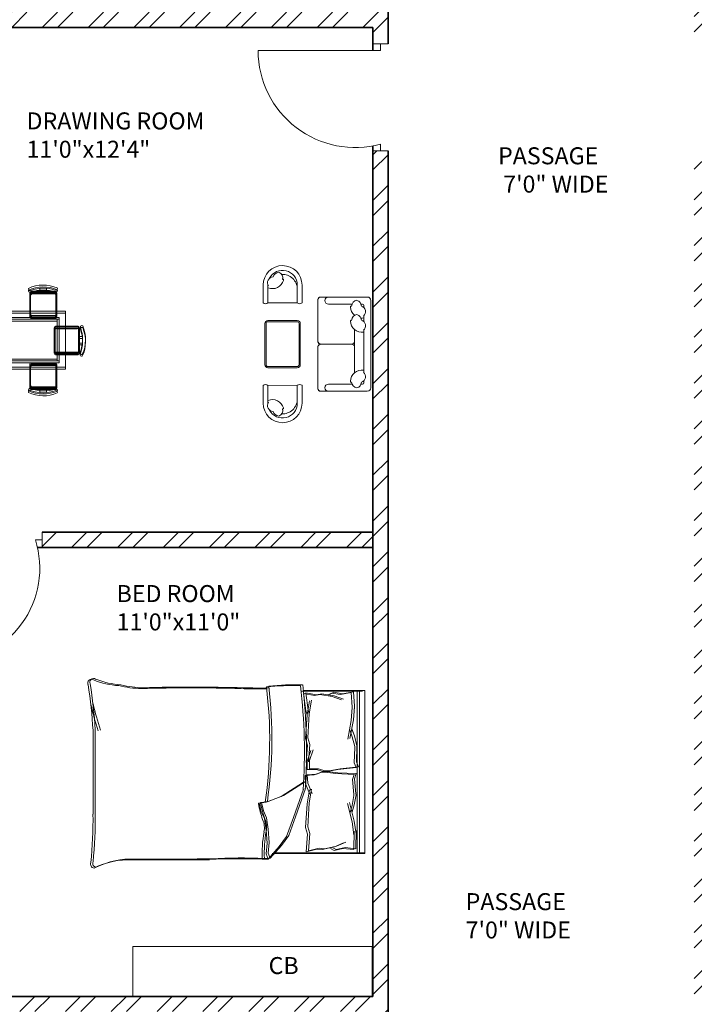
# Model space of a CAD drawing. Units: inches. Extents: x 2168 to 3056, y 1130 to 2629.
# Tile 5 of 42: x 2447 to 2645, y 1789 to 2079. Entities that reach past the tile are written whole.
import ezdxf

# ---------------------------------------------------------------- set-up
doc = ezdxf.new("R2010")
doc.units = ezdxf.units.IN
for name, color, linetype, lineweight in [('A-ANNO-TEXT', 7, 'Continuous', 18), ('A-AREA-IDEN', 7, 'Continuous', 18), ('A-DOOR', 21, 'Continuous', 18), ('A-FLOR-CASE', 71, 'Continuous', 18), ('A-FURN', 8, 'Continuous', 13), ('A-WALL', 7, 'Continuous', 35)]:
    doc.layers.add(name, color=color, linetype=linetype, lineweight=lineweight)
doc.layers.add('A-WALL-PATT', color=143, linetype='Continuous', lineweight=13, true_color=0x7aafdf)
doc.styles.get("Standard").update_dxf_attribs({"font": 'arial.ttf'})

# ---------------------------------------------------------------- blocks, each defined once
blk = doc.blocks.new('A$C1352')
at = {"color": 0}
for points in [[(0.003, 0.053), (0.003, 0.553, -0.414214), (0.053, 0.603), (0.753, 0.603, -0.414214), (0.803, 0.553), (0.803, 0.053, -0.414214), (0.753, 0.003), (0.053, 0.003, -0.414214)], [(0.023, 0.053), (0.023, 0.553, -0.414214), (0.053, 0.583), (0.753, 0.583, -0.414214), (0.783, 0.553), (0.783, 0.053, -0.414214), (0.753, 0.023), (0.053, 0.023, -0.414214)]]:
    blk.add_lwpolyline(points, format="xyb", close=True, dxfattribs=at)
blk = doc.blocks.new('BED-DOUBLE')
for p, q in [((27.75, 52.87), (24.5, 49.16)), ((27.75, 52.87), (24.5, 49.16)), ((28.39, 53.1), (25.14, 49.39)), ((28.39, 53.1), (25.14, 49.39)), ((29.49, 52.95), (27.75, 52.87, 3.87)), ((29.49, 52.95), (27.75, 52.87, 3.87)), ((28.37, 51.33), (27.75, 52.87)), ((28.37, 51.33), (27.75, 52.87)), ((30.13, 53.18), (28.39, 53.1, 3.87)), ((30.13, 53.18), (28.39, 53.1, 3.87)), ((29, 51.56), (28.39, 53.1)), ((29, 51.56), (28.39, 53.1)), ((0, 51.49), (0.64, 51.49)), ((0, 3.48), (0, 51.49)), ((0, 51.27), (26.61, 51.27)), ((0, 51.27), (26.61, 51.27)), ((0.64, 51.49), (27.25, 51.49)), ((0.64, 51.49), (27.25, 51.49)), ((1.53, 3.48), (1.53, 51.27)), ((1.53, 3.48), (1.53, 51.27)), ((2.17, 3.7), (2.17, 51.49)), ((2.17, 3.7), (2.17, 51.49)), ((2.56, 50.11), (2.46, 44.71)), ((2.56, 50.11), (2.46, 44.71)), ((2.56, 50.11), (5.77, 49.73)), ((2.56, 50.11), (5.77, 49.73)), ((3.2, 50.34), (3.1, 44.94)), ((3.2, 50.34), (3.1, 44.94)), ((3.2, 50.34), (6.41, 49.96)), ((3.2, 50.34), (6.41, 49.96)), ((8.26, 49.31), (5.58, 48.13)), ((8.26, 49.31), (5.58, 48.13)), ((5.77, 49.73), (8.34, 50.33)), ((5.77, 49.73), (8.34, 50.33)), ((8.9, 49.54), (6.22, 48.36)), ((8.9, 49.54), (6.22, 48.36)), ((6.41, 49.96), (8.98, 50.56)), ((6.41, 49.96), (8.98, 50.56)), ((11.83, 50.11), (8.26, 49.31)), ((11.83, 50.11), (8.26, 49.31)), ((8.34, 50.33), (9.38, 49.81)), ((8.34, 50.33), (9.38, 49.81)), ((12.47, 50.34), (8.9, 49.54)), ((12.47, 50.34), (8.9, 49.54)), ((8.98, 50.56), (10.02, 50.04)), ((8.98, 50.56), (10.02, 50.04)), ((13.43, 49.92), (11.83, 50.11)), ((13.43, 49.92), (11.83, 50.11)), ((14.07, 50.15), (12.47, 50.34)), ((14.07, 50.15), (12.47, 50.34)), ((16.57, 50.7), (13.43, 49.92)), ((16.57, 50.7), (13.43, 49.92)), ((17.21, 50.93), (14.07, 50.15)), ((17.21, 50.93), (14.07, 50.15)), ((16.17, 45.57), (16.57, 50.7)), ((16.17, 45.57), (16.57, 50.7)), ((16.81, 45.8), (17.21, 50.93)), ((16.81, 45.79), (17.21, 50.93)), ((25.14, 49.39), (22.97, 46.45)), ((25.14, 49.39), (22.97, 46.45)), ((28.06, 48.23), (28.37, 51.33)), ((28.06, 48.23), (28.37, 51.33)), ((28.7, 48.46), (29, 51.56)), ((28.7, 48.46), (29, 51.56)), ((22.97, 46.45), (20.96, 40.87)), ((22.97, 46.45), (20.96, 40.87)), ((24.5, 49.16), (22.33, 46.22)), ((24.5, 49.16), (22.33, 46.22)), ((28.37, 44.36), (28.06, 48.23)), ((28.37, 44.36), (28.06, 48.23)), ((29, 44.59), (28.7, 48.46)), ((29, 44.59), (28.7, 48.46)), ((2.46, 44.71), (2.54, 45.71)), ((2.46, 44.71), (2.54, 45.71)), ((2.54, 45.71), (3.07, 41.91)), ((2.54, 45.71), (3.07, 41.91)), ((3.1, 44.94), (3.18, 45.94)), ((3.1, 44.94), (3.18, 45.94)), ((3.18, 45.94), (3.71, 42.14)), ((3.18, 45.94), (3.71, 42.14)), ((16.73, 43.61), (16.17, 45.57)), ((16.73, 43.61), (16.17, 45.57)), ((16.3, 36.6), (16.73, 43.61)), ((16.3, 36.6), (16.73, 43.61)), ((17.37, 43.83), (16.81, 45.8)), ((17.37, 43.83), (16.81, 45.79)), ((16.93, 36.82), (17.37, 43.83)), ((16.93, 36.82), (17.37, 43.83)), ((22.33, 46.22), (20.32, 40.64)), ((22.33, 46.22), (20.32, 40.64)), ((28.83, 40.95), (28.37, 44.36)), ((28.83, 40.95), (28.37, 44.36)), ((29.47, 41.18), (29, 44.59)), ((29.47, 41.18), (29, 44.59)), ((3.07, 41.91), (4.42, 36.5)), ((3.07, 41.91), (4.42, 36.49)), ((3.71, 42.14), (5.06, 36.72)), ((3.71, 42.14), (5.06, 36.72)), ((20.32, 40.64), (17.38, 32.31)), ((20.32, 40.64), (17.38, 32.31)), ((20.96, 40.87), (18.02, 32.53)), ((20.96, 40.87), (18.02, 32.53)), ((29.76, 38.94), (28.83, 40.95)), ((29.76, 38.94), (28.83, 40.95)), ((30.4, 39.17), (29.47, 41.18)), ((30.4, 39.17), (29.47, 41.18)), ((3.67, 39.2), (3.08, 37.14)), ((3.67, 39.2), (3.08, 37.14)), ((4.31, 39.43), (3.72, 37.36)), ((4.31, 39.43), (3.72, 37.36)), ((30.38, 36.46), (29.76, 38.94)), ((30.38, 36.46), (29.76, 38.94)), ((31.02, 36.69), (30.4, 39.17)), ((31.02, 36.69), (30.4, 39.17)), ((79.25, 15.06), (79.25, 39.68)), ((79.25, 15.06), (79.25, 39.68)), ((79.88, 15.29), (79.88, 39.91)), ((79.88, 15.29), (79.88, 39.91)), ((3.08, 37.14), (2.54, 34.2)), ((3.08, 37.14), (2.54, 34.2)), ((3.72, 37.36), (3.18, 34.43)), ((3.72, 37.36), (3.18, 34.43)), ((15.63, 32.56), (16.3, 36.6)), ((15.63, 32.56), (16.3, 36.6)), ((16.27, 32.79), (16.93, 36.82)), ((16.27, 32.79), (16.93, 36.82)), ((23.88, 34.45), (28.37, 36.15)), ((23.88, 34.45), (28.37, 36.15)), ((24.52, 34.68), (29, 36.38)), ((24.52, 34.68), (29, 36.38)), ((28.37, 36.15), (30.38, 36.46)), ((28.37, 36.15), (30.38, 36.46)), ((29, 36.38), (31.02, 36.69)), ((29, 36.38), (31.02, 36.69)), ((2.54, 34.2), (2.56, 33.88)), ((2.54, 34.2), (2.56, 33.88)), ((2.56, 33.88), (2.98, 29.46)), ((2.56, 33.88), (2.98, 29.46)), ((3.18, 34.43), (3.2, 34.11)), ((3.18, 34.43), (3.2, 34.11)), ((3.2, 34.11), (3.62, 29.68)), ((3.2, 34.11), (3.62, 29.68)), ((16.74, 30.75), (15.45, 33.82)), ((16.74, 30.75), (15.45, 33.82)), ((17.38, 30.98), (16.09, 34.05)), ((17.38, 30.98), (16.09, 34.05)), ((17.38, 30.26), (23.88, 34.45)), ((17.38, 30.26), (23.88, 34.45)), ((18.02, 30.49), (24.52, 34.68)), ((18.02, 30.49), (24.52, 34.68)), ((2.98, 29.46), (2.49, 27.98)), ((2.98, 29.46), (2.49, 27.98)), ((3.62, 29.68), (3.13, 28.21)), ((3.62, 29.68), (3.13, 28.21)), ((16.89, 28.3), (16.74, 30.75)), ((16.89, 28.3), (16.74, 30.75)), ((17.53, 28.53), (17.38, 30.98)), ((17.53, 28.53), (17.38, 30.98)), ((1.87, 25.98), (7.22, 26.56)), ((1.87, 25.98), (7.22, 26.56)), ((2.49, 27.98), (7.87, 27.73)), ((2.49, 27.98), (7.87, 27.73)), ((2.51, 26.21), (7.86, 26.79)), ((2.51, 26.21), (7.86, 26.79)), ((3.09, 24.77), (2.51, 26.21)), ((3.09, 24.77), (2.51, 26.21)), ((3.13, 28.21), (8.51, 27.96)), ((3.13, 28.21), (8.51, 27.96)), ((7.22, 26.56), (10.4, 27.14)), ((7.22, 26.56), (10.4, 27.14)), ((7.86, 26.79), (11.04, 27.37)), ((7.86, 26.79), (11.04, 27.37)), ((7.87, 27.73), (11.08, 27.36)), ((7.87, 27.73), (11.08, 27.35)), ((8.51, 27.96), (11.72, 27.58)), ((8.51, 27.96), (11.72, 27.58)), ((10.4, 27.14), (11.7, 27.14)), ((10.4, 27.14), (11.7, 27.14)), ((11.04, 27.37), (12.34, 27.37)), ((11.04, 27.37), (12.34, 27.37)), ((11.08, 27.36), (12.38, 27.44)), ((11.08, 27.35), (12.38, 27.44)), ((11.7, 27.14), (13.58, 26.56)), ((11.7, 27.14), (13.58, 26.56)), ((11.72, 27.58), (13.02, 27.66)), ((11.72, 27.58), (13.02, 27.66)), ((12.34, 27.37), (14.22, 26.79)), ((12.34, 27.37), (14.22, 26.79)), ((12.38, 27.44), (14.22, 28.13)), ((12.38, 27.44), (14.22, 28.13)), ((13.02, 27.66), (14.86, 28.36)), ((13.02, 27.66), (14.86, 28.36)), ((13.58, 26.56), (16.26, 26.56)), ((13.58, 26.56), (16.26, 26.56)), ((14.22, 28.13), (16.89, 28.3)), ((14.22, 28.13), (16.89, 28.3)), ((14.22, 26.79), (16.9, 26.79)), ((14.22, 26.79), (16.9, 26.79)), ((14.86, 28.36), (17.53, 28.53)), ((14.86, 28.36), (17.53, 28.53)), ((16.26, 26.56), (16.26, 24.1)), ((16.26, 26.56), (16.26, 24.1)), ((16.9, 26.79), (16.9, 24.33)), ((16.9, 26.79), (16.9, 24.33)), ((2.45, 24.54), (1.87, 25.98)), ((2.45, 24.54), (1.87, 25.98)), ((2.3, 20.09), (2.45, 24.54)), ((2.3, 20.09), (2.45, 24.54)), ((2.94, 20.32), (3.09, 24.77)), ((2.94, 20.32), (3.09, 24.77)), ((16.26, 24.1), (15.17, 20.96)), ((16.26, 24.1), (15.17, 20.96)), ((16.9, 24.33), (15.81, 21.19)), ((16.9, 24.33), (15.81, 21.19)), ((16.17, 19.38), (16.57, 24.52)), ((16.17, 19.38), (16.57, 24.52)), ((16.81, 19.61), (17.21, 24.74)), ((16.81, 19.61), (17.21, 24.74)), ((2.94, 20), (2.94, 20.32)), ((2.94, 20), (2.94, 20.32)), ((2.3, 19.77), (2.3, 20.09)), ((2.3, 19.77), (2.3, 20.09)), ((3.03, 16.88), (2.3, 19.77)), ((3.03, 16.88), (2.3, 19.77)), ((3.67, 17.11), (2.94, 20)), ((3.67, 17.11), (2.94, 20)), ((3.32, 12.11), (4.33, 17.6)), ((3.32, 12.11), (4.33, 17.6)), ((3.96, 12.34), (4.97, 17.83)), ((3.96, 12.34), (4.97, 17.83)), ((16.73, 17.42), (16.17, 19.38)), ((16.73, 17.42), (16.17, 19.38)), ((16.3, 10.41), (16.73, 17.42)), ((16.3, 10.41), (16.73, 17.42)), ((17.37, 17.65), (16.81, 19.61)), ((17.37, 17.65), (16.81, 19.61)), ((16.93, 10.64), (17.37, 17.65)), ((16.93, 10.64), (17.37, 17.65)), ((3.75, 14.86), (3.03, 16.88)), ((3.75, 14.85), (3.03, 16.88)), ((4.39, 15.08), (3.67, 17.11)), ((4.39, 15.08), (3.67, 17.11)), ((3.03, 8.29), (3.32, 12.11)), ((3.03, 8.28), (3.32, 12.11)), ((3.67, 8.51), (3.96, 12.34)), ((3.67, 8.51), (3.96, 12.34)), ((15.63, 6.38), (16.3, 10.41)), ((15.63, 6.38), (16.3, 10.41)), ((16.27, 6.61), (16.93, 10.64)), ((16.27, 6.61), (16.93, 10.64)), ((16.3, 10.41), (16.62, 9.28)), ((16.3, 10.41), (16.62, 9.28)), ((16.62, 9.28), (17.34, 4.18)), ((16.62, 9.28), (17.34, 4.18)), ((16.93, 10.64), (17.26, 9.51)), ((16.93, 10.64), (17.26, 9.51)), ((17.26, 9.51), (17.98, 4.41)), ((17.26, 9.51), (17.98, 4.41)), ((3.01, 8.18), (3.03, 8.29)), ((3.01, 8.18), (3.03, 8.28)), ((3.34, 3.9), (3.01, 8.18)), ((3.34, 3.9), (3.01, 8.18)), ((3.65, 8.41), (3.67, 8.51)), ((3.65, 8.41), (3.67, 8.51)), ((3.98, 4.13), (3.65, 8.41)), ((3.98, 4.13), (3.65, 8.41)), ((8.96, 5.05), (6.21, 6.06)), ((8.96, 5.05), (6.21, 6.06)), ((9.59, 5.28), (6.85, 6.29)), ((9.59, 5.28), (6.85, 6.29)), ((18.11, 3.48), (0, 3.48)), ((18.11, 3.48), (0, 3.48)), ((18.75, 3.7), (0.64, 3.7)), ((18.75, 3.7), (0.64, 3.7)), ((3.32, 3.89), (6.5, 4.47)), ((3.32, 3.89), (6.5, 4.47)), ((3.96, 4.12), (7.14, 4.7)), ((3.96, 4.12), (7.14, 4.7)), ((6.5, 4.47), (9.1, 4.04)), ((6.5, 4.47), (9.1, 4.04)), ((7.14, 4.7), (9.74, 4.27)), ((7.14, 4.7), (9.74, 4.27)), ((12.57, 4.47), (8.96, 5.05)), ((12.57, 4.47), (8.96, 5.05)), ((9.1, 4.04), (10.11, 4.62)), ((9.1, 4.04), (10.11, 4.62)), ((13.21, 4.7), (9.59, 5.28)), ((13.21, 4.7), (9.59, 5.28)), ((9.74, 4.27), (10.75, 4.85)), ((9.74, 4.27), (10.75, 4.85)), ((14.16, 4.76), (12.57, 4.47)), ((14.16, 4.76), (12.57, 4.47)), ((14.8, 4.99), (13.21, 4.7)), ((14.8, 4.99), (13.21, 4.7)), ((17.34, 4.18), (14.16, 4.76)), ((17.34, 4.18), (14.16, 4.76)), ((17.98, 4.41), (14.8, 4.99)), ((17.98, 4.41), (14.8, 4.99))]:
    blk.add_line(p, q)
for centre, radius, start, end in [((68.67, 76.16), 23.07, 267.4714, 296.4681), ((68.67, 76.16), 23.07, 267.4714, 296.4681), ((69.31, 76.39), 23.07, 267.4714, 296.4681), ((69.31, 76.39), 23.07, 267.4714, 296.4681), ((78.87, 54.41), 1.1, 332.6588, 86.02), ((78.87, 54.41), 1.1, 332.6588, 86.02), ((79.51, 54.64), 1.1, 332.6588, 86.02), ((79.51, 54.64), 1.1, 332.6588, 86.02), ((-6.66, 51.33), 36.18, 349.8763, 2.5657), ((-6.66, 51.33), 36.18, 349.8763, 2.5657), ((36.32, 182.27), 129.5, 266.9791, 273.8365), ((36.32, 182.27), 129.5, 266.9791, 273.8365), ((-6.02, 51.56), 36.18, 349.8763, 2.5657), ((-6.02, 51.56), 36.18, 349.8763, 2.5657), ((36.95, 182.49), 129.5, 266.9791, 273.8365), ((36.95, 182.49), 129.5, 266.9791, 273.8365), ((67.82, -4508.74), 4561.86, 90.00217, 90.28689), ((67.82, -4508.74), 4561.86, 90.00217, 90.28689), ((68.46, -4508.51), 4561.86, 90.00217, 90.28689), ((68.46, -4508.52), 4561.86, 90.00217, 90.28689), ((212.28, 41.15), 133.04, 174.4998, 180.6351), ((212.28, 41.15), 133.04, 174.4998, 180.6351), ((212.92, 41.38), 133.04, 174.4998, 180.6351), ((212.92, 41.38), 133.04, 174.4998, 180.6351), ((35.07, 43.74), 6.22, 168.6608, 203.7384), ((35.07, 43.74), 6.22, 168.6608, 203.7384), ((35.71, 43.97), 6.22, 168.6608, 203.7384), ((35.71, 43.97), 6.22, 168.6608, 203.7384), ((1.48, 31.15), 29.65, 10.6617, 19.8806), ((1.48, 31.15), 29.65, 10.6617, 19.8806), ((2.12, 31.38), 29.65, 10.6617, 19.8806), ((2.12, 31.38), 29.65, 10.6617, 19.8806), ((156.32, 17.76), 129.02, 171.7845, 186.9006), ((156.32, 17.76), 129.02, 171.7845, 186.9006), ((156.96, 17.98), 129.02, 171.7845, 186.9006), ((156.96, 17.98), 129.02, 171.7845, 186.9006), ((30.44, 36.64), 0.185, 250.2464, 1.1377), ((30.44, 36.64), 0.185, 250.2464, 1.1377), ((31.08, 36.86), 0.185, 250.2464, 1.1377), ((31.08, 36.86), 0.185, 250.2464, 1.1377), ((182.05, 21.36), 164.97, 176.0865, 186.7821), ((182.05, 21.36), 164.97, 176.0865, 186.7821), ((182.69, 21.59), 164.97, 176.0865, 186.7821), ((182.69, 21.59), 164.97, 176.0865, 186.7821), ((-23.71, -17.22), 106.46, 13.3832, 17.7053), ((-23.71, -17.22), 106.46, 13.3832, 17.7053), ((-23.07, -16.99), 106.46, 13.3832, 17.7053), ((-23.07, -16.99), 106.46, 13.3832, 17.7053), ((200.84, 21.43), 121.76, 182.9958, 189.4091), ((200.84, 21.43), 121.76, 182.9958, 189.4091), ((201.48, 21.66), 121.76, 182.9958, 189.4091), ((201.48, 21.66), 121.76, 182.9958, 189.4091), ((31.81, -167.08), 170.11, 88.4762, 91.0082), ((31.81, -167.08), 170.11, 88.4762, 91.0082), ((51.25, 485.05), 482.31, 268.2277, 271.7185), ((51.25, 485.05), 482.31, 268.2277, 271.7185), ((65.15, -26.67), 29.63, 76.0648, 88.9113), ((65.15, -26.67), 29.63, 76.0648, 88.9113), ((20.1, 85.16), 83.31, 268.7218, 275.604), ((20.1, 85.16), 83.31, 268.7218, 275.604), ((20.74, 85.39), 83.31, 268.7218, 275.604), ((20.74, 85.39), 83.31, 268.7218, 275.604), ((31.17, -167.31), 170.11, 88.4762, 91.0082), ((31.17, -167.31), 170.11, 88.4762, 91.0082), ((50.61, 484.82), 482.31, 268.2277, 271.7185), ((50.61, 484.82), 482.31, 268.2277, 271.7185), ((64.52, -26.9), 29.63, 76.0648, 88.9113), ((64.52, -26.9), 29.63, 76.0648, 88.9113), ((70.28, -21.66), 23.56, 67.9751, 86.652), ((70.28, -21.66), 23.56, 67.9751, 86.652), ((70.92, -21.43), 23.56, 67.9751, 86.652), ((70.92, -21.43), 23.56, 67.9751, 86.652), ((79.72, 1.09), 1.09, 236.1736, 23.4781), ((79.72, 1.09), 1.09, 236.1736, 23.4781), ((80.36, 1.32), 1.09, 236.1736, 23.4781), ((80.36, 1.32), 1.09, 236.1736, 23.4781)]:
    blk.add_arc(centre, radius, start, end)
blk = doc.blocks.new('CHAIR-LOUNGE')
blk.add_line((10.04, 5.71), (10.04, 10.98))
at = {"ltscale": 0.03}
blk.add_lwpolyline([(10.04, 10.98, -0.369229), (11.42, 10.98), (11.42, 5.7, -1), (0, 5.72), (0, 10.99, -0.369229), (1.39, 10.99)], format="xyb", close=True, dxfattribs=at)
blk.add_lwpolyline([(9.55, 3.71, -0.785087), (1.38, 5.71), (1.39, 10.99)], format="xyb")
for centre, radius, start, end in [((5.71, 6.93), 4.33, 179.9461, 273.658), ((8.67, 3.43), 3.35, 67.0143, 164.2857), ((8.41, 5.02), 1.73, 272.9922, 34.1401), ((5.63, 4.23), 0.207, 150.6238, 293.7423), ((7.44, 3.63), 1.78, 166.6403, 249.4695), ((6.65, 3.91), 1.95, 274.9999, 341.3534), ((5.71, 5.71), 4.33, 358.8536, 359.9461)]:
    blk.add_arc(centre, radius, start, end)
blk = doc.blocks.new('TABLE-DINING')
for points in [[(0, 17.02), (27.45, 17.02), (27.45, 0.55), (0, 0.55)], [(0, 17.02), (27.45, 17.02), (27.45, 0.55), (0, 0.55)], [(0, 16.47), (27.45, 16.47), (27.45, 0), (0, 0)], [(0, 16.47), (27.45, 16.47), (27.45, 0), (0, 0)], [(1.83, 15.19), (25.62, 15.19), (25.62, 2.38), (1.83, 2.38)], [(1.83, 15.19), (25.62, 15.19), (25.62, 2.38), (1.83, 2.38)], [(1.83, 14.64), (25.62, 14.64), (25.62, 1.83), (1.83, 1.83)], [(1.83, 14.64), (25.62, 14.64), (25.62, 1.83), (1.83, 1.83)], [(2.38, 14.64), (25.07, 14.64), (25.07, 2.93), (2.38, 2.93)], [(2.38, 14.64), (25.07, 14.64), (25.07, 2.93), (2.38, 2.93)], [(2.38, 14.09), (25.07, 14.09), (25.07, 2.38), (2.38, 2.38)], [(2.38, 14.09), (25.07, 14.09), (25.07, 2.38), (2.38, 2.38)]]:
    blk.add_lwpolyline(points, close=True)
blk = doc.blocks.new('CUPBOARD-BEDROOM')
blk.add_lwpolyline([(0, 14.89), (70.36, 14.89), (70.36, 0), (0, 0)], close=True)

msp = doc.modelspace()

# ---------------------------------------------------------------- hatches: boundary and pattern name
at = {"layer": 'A-WALL-PATT'}
h = msp.add_hatch(dxfattribs=at)
h.set_pattern_fill('ANSI32', color=256)
h.paths.add_polyline_path([(2463.8, 2409.39), (2467.39, 2409.39), (2467.39, 2413.89), (2454.77, 2413.89), (2454.77, 2411.64), (2454.77, 2409.39), (2459.3, 2409.39), (2459.3, 2265.39), (2455.64, 2265.39), (2455.64, 2260.89), (2467.35, 2260.89), (2467.35, 2263.14), (2467.35, 2265.39), (2463.8, 2265.39)])
h.paths.add_polyline_path([(2431.6, 2413.89), (2409.65, 2413.89), (2409.65, 2409.39), (2431.6, 2409.39), (2431.6, 2411.64)])
h.paths.add_polyline_path([(2349.65, 2413.89), (2331.8, 2413.89), (2331.8, 2362.67), (2336.3, 2362.67), (2336.3, 2409.39), (2349.65, 2409.39), (2349.65, 2411.64)])
h.paths.add_polyline_path([(2634.15, 2411.64), (2634.15, 2413.89), (2562.29, 2413.89), (2562.29, 2409.39), (2595.8, 2409.39), (2595.8, 2280.31), (2595.83, 2280.31), (2595.83, 2265.39), (2499.91, 2265.39), (2499.91, 2260.89), (2550.8, 2260.89), (2550.8, 2117.31), (2555.3, 2117.31), (2555.3, 2168.08), (2571.93, 2168.08), (2571.93, 2176.89), (2559.8, 2176.89), (2559.8, 2256.39), (2640.8, 2256.39), (2640.8, 2176.89), (2626.43, 2176.89), (2626.43, 2168.08), (2645.3, 2168.08), (2645.3, 2116.64), (2649.8, 2116.64), (2649.8, 2260.89), (2691.25, 2260.89), (2691.25, 2263.14), (2691.25, 2265.39), (2670.65, 2265.39), (2670.65, 2265.36), (2600.3, 2265.36), (2600.3, 2280.26), (2600.3, 2409.39), (2634.15, 2409.39)])
h.paths.add_polyline_path([(2600.3, 2473.89), (2612.84, 2473.89), (2612.84, 2478.39), (2572.64, 2478.39), (2572.64, 2473.89), (2595.8, 2473.89), (2595.8, 2413.89), (2600.3, 2413.89)])
h.paths.add_polyline_path([(2535.8, 2473.89), (2548.64, 2473.89), (2548.64, 2478.39), (2531.4, 2478.39), (2531.4, 2413.89), (2521.6, 2413.89), (2521.6, 2409.39), (2539.24, 2409.39), (2539.24, 2411.64), (2539.24, 2413.89), (2535.8, 2413.89)])
h.paths.add_polyline_path([(2664.8, 2478.39), (2636.84, 2478.39), (2636.84, 2473.89), (2660.3, 2473.89), (2660.3, 2413.89), (2656.17, 2413.89), (2656.17, 2409.39), (2671.68, 2409.39), (2671.68, 2411.64), (2671.68, 2413.89), (2664.8, 2413.89)])
h.paths.add_polyline_path([(2705.94, 2413.89), (2695.68, 2413.89), (2695.68, 2409.39), (2705.94, 2409.39)])
h.paths.add_polyline_path([(2741.35, 2413.89), (2728.73, 2413.89), (2728.73, 2411.64), (2728.73, 2409.39), (2732.3, 2409.39), (2732.3, 2265.39), (2725.73, 2265.39), (2725.73, 2260.89), (2740.92, 2260.89), (2740.92, 2263.14), (2740.92, 2265.39), (2736.8, 2265.39), (2736.8, 2409.39), (2741.35, 2409.39)])
h.paths.add_polyline_path([(2785.65, 2413.89), (2764.55, 2413.89), (2764.49, 2409.39), (2785.65, 2409.39), (2785.65, 2411.64)])
h.paths.add_polyline_path([(2864.3, 2413.89), (2845.65, 2413.89), (2845.65, 2409.39), (2859.8, 2409.39), (2859.8, 2368.43), (2864.3, 2368.43)])
h.paths.add_polyline_path([(2864.3, 2308.43), (2862.05, 2308.43), (2859.8, 2308.43), (2859.8, 2265.39), (2774.48, 2265.39), (2774.48, 2263.14), (2774.48, 2260.89), (2781.8, 2260.89), (2781.8, 2226.65), (2786.3, 2226.65), (2786.3, 2260.89), (2859.8, 2260.89), (2859.8, 2241.35), (2864.3, 2241.35)])
h.paths.add_polyline_path([(2864.3, 2217.35), (2862.05, 2217.35), (2859.8, 2217.35), (2859.8, 2200.89), (2786.3, 2200.89), (2786.3, 2205.93), (2784.05, 2205.93), (2781.8, 2205.93), (2781.8, 2150.97), (2786.3, 2150.97), (2786.3, 2161.89), (2859.8, 2161.89), (2859.8, 2144.42), (2864.3, 2144.42)])
h.paths.add_polyline_path([(2859.8, 2196.39), (2859.8, 2166.39), (2786.3, 2166.39), (2786.3, 2196.39)], flags=16)
h.paths.add_polyline_path([(2864.3, 2108.42), (2862.05, 2108.42), (2859.8, 2108.42), (2859.8, 2080.89), (2786.3, 2080.89), (2786.3, 2111.99), (2781.8, 2111.99), (2781.8, 2080.89), (2649.8, 2080.89), (2649.8, 2086.04), (2647.55, 2086.04), (2645.3, 2086.04), (2645.3, 2071.74), (2649.8, 2071.74), (2649.8, 2076.39), (2781.8, 2076.39), (2781.8, 2041.79), (2786.3, 2041.79), (2786.3, 2076.39), (2859.8, 2076.39), (2859.8, 2058.58), (2864.3, 2058.58)])
h.paths.add_polyline_path([(2864.3, 2022.58), (2859.8, 2022.58), (2859.8, 1992.39), (2786.3, 1992.39), (2786.3, 1999.57), (2781.8, 1999.57), (2781.8, 1848.09), (2784.05, 1848.09), (2786.3, 1848.09), (2786.3, 1851.39), (2859.8, 1851.39), (2859.8, 1838.26), (2864.3, 1838.26)], flags=17)
h.paths.add_polyline_path([(2859.8, 1987.89), (2859.8, 1855.89), (2786.3, 1855.89), (2786.3, 1987.89)], flags=16)
h.paths.add_polyline_path([(2823.05, 1987.89), (2841.42, 1921.89), (2823.05, 1855.89)], flags=0)
h.paths.add_polyline_path([(2864.3, 1814.26), (2859.8, 1814.26), (2859.8, 1791.39), (2786.3, 1791.39), (2786.3, 1825.66), (2784.05, 1825.66), (2781.8, 1825.66), (2781.8, 1791.39), (2720.15, 1791.39), (2720.15, 1791.27), (2649.8, 1791.27), (2649.8, 1806.16), (2649.8, 2038.98), (2647.55, 2038.98), (2645.3, 2038.98), (2645.3, 1783.93), (2649.8, 1783.93), (2649.8, 1786.89), (2781.8, 1786.89), (2781.8, 1746.79), (2786.3, 1746.79), (2786.3, 1786.89), (2859.8, 1786.89), (2859.8, 1770.08), (2864.3, 1770.08)])
h.paths.add_polyline_path([(2864.3, 1734.08), (2862.05, 1734.08), (2859.8, 1734.08), (2859.8, 1705.89), (2786.3, 1705.89), (2786.3, 1714.17), (2781.8, 1714.17), (2781.8, 1660.53), (2786.3, 1660.53), (2786.3, 1666.89), (2859.8, 1666.89), (2859.8, 1648.34), (2864.3, 1648.34)])
h.paths.add_polyline_path([(2786.3, 1701.39), (2859.8, 1701.39), (2859.8, 1671.39), (2786.3, 1671.39)], flags=16)
h.paths.add_polyline_path([(2649.8, 1756.58), (2647.55, 1756.58), (2645.3, 1756.58), (2645.3, 1606.89), (2555.3, 1606.89), (2555.3, 1749.51), (2553.05, 1749.51), (2550.8, 1749.51), (2550.8, 1606.89), (2503.01, 1606.89), (2503.01, 1604.64), (2503.01, 1602.39), (2595.8, 1602.39), (2595.85, 1602.39), (2595.85, 1587.5), (2595.8, 1458.39), (2561.5, 1458.39), (2561.5, 1456.14), (2561.5, 1453.89), (2595.8, 1453.89), (2595.8, 1381.89), (2573.44, 1381.89), (2573.44, 1377.39), (2613.01, 1377.39), (2613.01, 1379.64), (2613.01, 1381.89), (2600.3, 1381.89), (2600.3, 1453.89), (2634.33, 1453.89), (2634.33, 1458.39), (2600.3, 1458.39), (2600.3, 1602.39), (2670.65, 1602.39), (2694.09, 1602.39), (2694.09, 1606.89), (2649.8, 1606.89)])
h.paths.add_polyline_path([(2736.8, 1602.39), (2741.56, 1602.39), (2741.56, 1606.89), (2726.2, 1606.89), (2726.2, 1604.64), (2726.2, 1602.39), (2732.3, 1602.39), (2732.3, 1458.39), (2727.9, 1458.39), (2727.9, 1453.89), (2740.82, 1453.89), (2740.82, 1456.14), (2740.82, 1458.39), (2736.8, 1458.39)])
h.paths.add_polyline_path([(2859.8, 1606.89), (2786.3, 1606.89), (2786.3, 1637.33), (2784.05, 1637.33), (2781.8, 1637.33), (2781.8, 1606.89), (2775.61, 1606.89), (2775.61, 1602.39), (2859.8, 1602.39)])
h.paths.add_polyline_path([(2864.3, 1624.34), (2862.05, 1624.34), (2859.8, 1624.34), (2859.8, 1570.39), (2864.3, 1570.39)])
h.paths.add_polyline_path([(2864.3, 1510.39), (2862.05, 1510.39), (2859.8, 1510.39), (2859.8, 1458.39), (2846.73, 1458.39), (2846.73, 1456.14), (2846.73, 1453.89), (2864.3, 1453.89)])
h.paths.add_polyline_path([(2786.73, 1458.39), (2765.44, 1458.39), (2765.44, 1453.89), (2786.73, 1453.89)])
h.paths.add_polyline_path([(2706, 1458.39), (2695.36, 1458.39), (2695.36, 1453.89), (2706, 1453.89), (2706, 1456.14)])
h.paths.add_polyline_path([(2671.36, 1456.14), (2671.36, 1458.39), (2655.99, 1458.39), (2655.99, 1456.14), (2655.99, 1453.89), (2660.3, 1453.89), (2660.3, 1381.89), (2637.01, 1381.89), (2637.01, 1377.39), (2664.8, 1377.39), (2664.8, 1453.89), (2671.36, 1453.89)], flags=17)
h.paths.add_polyline_path([(2539.83, 1458.39), (2520.24, 1458.39), (2520.24, 1453.89), (2531.3, 1453.89), (2531.3, 1377.39), (2546.45, 1377.39), (2546.45, 1379.64), (2546.45, 1381.89), (2535.8, 1381.89), (2535.8, 1453.89), (2539.83, 1453.89)], flags=17)
h.paths.add_polyline_path([(2496.24, 1458.39), (2489.13, 1458.39), (2489.13, 1453.89), (2496.24, 1453.89), (2496.24, 1456.14)])
h.paths.add_polyline_path([(2467.43, 1456.14), (2467.43, 1458.39), (2463.8, 1458.39), (2463.8, 1602.39), (2468.24, 1602.39), (2468.24, 1605.7), (2468.24, 1606.89), (2454.6, 1606.89), (2454.6, 1602.39), (2459.3, 1602.39), (2459.3, 1458.39), (2454.24, 1458.39), (2454.24, 1453.89), (2467.43, 1453.89)])
h.paths.add_polyline_path([(2431.6, 1456.14), (2431.6, 1458.39), (2411.39, 1458.39), (2411.39, 1453.89), (2431.6, 1453.89)])
h.paths.add_polyline_path([(2351.39, 1458.39), (2336.3, 1458.39), (2336.3, 1490.69), (2334.05, 1490.69), (2331.8, 1490.69), (2331.8, 1453.89), (2351.39, 1453.89), (2351.39, 1456.14)])
h.paths.add_polyline_path([(2336.3, 1629.7), (2331.8, 1629.7), (2331.8, 1552.32), (2336.3, 1552.32), (2336.3, 1602.39), (2406.65, 1602.39), (2423.47, 1602.39), (2423.47, 1606.89), (2418.8, 1606.89), (2418.8, 1643.68), (2416.55, 1643.68), (2414.3, 1643.68), (2414.3, 1606.89), (2336.3, 1606.89)])
h.paths.add_polyline_path([(2418.8, 1714.38), (2414.3, 1714.38), (2414.3, 1705.89), (2336.3, 1705.89), (2336.3, 1731.32), (2334.05, 1731.32), (2331.8, 1731.32), (2331.8, 1653.7), (2334.05, 1653.7), (2336.3, 1653.7), (2336.3, 1666.89), (2414.3, 1666.89), (2414.3, 1663.59), (2418.8, 1663.59)])
h.paths.add_polyline_path([(2336.3, 1701.39), (2414.3, 1701.39), (2414.3, 1671.39), (2336.3, 1671.39)], flags=16)
h.paths.add_polyline_path([(2555.3, 2040.06), (2550.8, 2040.06), (2550.8, 1791.39), (2550.56, 1791.2), (2480.2, 1791.2), (2418.8, 1791.39), (2418.8, 1825.45), (2416.55, 1825.45), (2414.3, 1825.45), (2414.3, 1791.39), (2336.3, 1791.39), (2336.3, 1806.41), (2331.8, 1806.41), (2331.8, 1767.32), (2336.3, 1767.32), (2336.3, 1786.89), (2414.3, 1786.89), (2414.3, 1745.46), (2418.8, 1745.46), (2418.8, 1786.89), (2550.8, 1786.89), (2550.8, 1783.01), (2555.3, 1783.01)])
h.paths.add_polyline_path([(2418.8, 1923.39), (2423.21, 1923.39), (2423.21, 1925.64), (2423.21, 1927.89), (2418.8, 1927.89), (2418.8, 2000.05), (2414.3, 2000.05), (2414.3, 1992.39), (2336.3, 1992.39), (2336.3, 1987.89), (2414.3, 1987.89), (2414.3, 1855.89), (2336.3, 1855.89), (2336.3, 1851.39), (2414.3, 1851.39), (2414.3, 1846.76), (2418.8, 1846.76)], flags=17)
h.paths.add_polyline_path([(2336.3, 2019.29), (2334.05, 2019.29), (2331.8, 2019.29), (2331.8, 1830.41), (2336.3, 1830.41)], flags=17)
h.paths.add_polyline_path([(2550.8, 1927.89), (2453.54, 1927.89), (2453.54, 1925.64), (2453.54, 1923.39), (2550.8, 1923.39)], flags=17)
h.paths.add_polyline_path([(2744.99, 1927.89), (2649.8, 1927.89), (2649.8, 1923.39), (2744.99, 1923.39), (2744.99, 1925.64)], flags=17)
h.paths.add_polyline_path([(2555.3, 2086.46), (2553.05, 2086.46), (2550.8, 2086.46), (2550.8, 2080.89), (2418.8, 2080.89), (2336.3, 2080.89), (2336.3, 2115.4), (2334.05, 2115.4), (2331.8, 2115.4), (2331.8, 2055.29), (2336.3, 2055.29), (2336.3, 2076.39), (2550.8, 2076.39), (2550.8, 2071.54), (2555.3, 2071.54)])
h.paths.add_polyline_path([(2418.8, 2121.39), (2414.3, 2121.39), (2414.3, 2080.89), (2418.8, 2080.89)])
h.paths.add_polyline_path([(2418.8, 2076.39), (2414.3, 2076.39), (2414.3, 2035.12), (2418.8, 2035.12)])
h.paths.add_polyline_path([(2422.87, 2263.14), (2422.87, 2265.39), (2406.65, 2265.39), (2406.65, 2265.36), (2336.3, 2265.36), (2336.3, 2280.25), (2336.3, 2302.67), (2334.05, 2302.67), (2331.8, 2302.67), (2331.8, 2246.85), (2336.3, 2246.85), (2336.3, 2260.89), (2414.3, 2260.89), (2414.3, 2224), (2418.8, 2224), (2418.8, 2260.89), (2422.87, 2260.89)])
h.paths.add_polyline_path([(2418.8, 2204.78), (2416.55, 2204.78), (2414.3, 2204.78), (2414.3, 2200.89), (2336.3, 2200.89), (2336.3, 2220.85), (2331.8, 2220.85), (2331.8, 2151.4), (2336.3, 2151.4), (2336.3, 2161.89), (2414.3, 2161.89), (2414.3, 2153.73), (2418.8, 2153.73)])
h.paths.add_polyline_path([(2414.3, 2196.39), (2414.3, 2166.39), (2336.3, 2166.39), (2336.3, 2196.39)], flags=16)
h.paths.add_polyline_path([(2375.3, 2181.39), (2336.3, 2166.39), (2336.3, 2196.39)], flags=0)
h.paths.add_polyline_path([(2809.6, 2172.34), (2838.8, 2172.34), (2838.8, 2191), (2809.6, 2191)], flags=8)
h.paths.add_polyline_path([(2849.75, 1919.59), (2849.75, 1952.67), (2831.09, 1952.67), (2831.09, 1919.59)], flags=8)
h.paths.add_polyline_path([(2808.87, 1901.97), (2808.87, 1937.85), (2790.15, 1937.85), (2790.15, 1901.97)], flags=8)
h.paths.add_polyline_path([(2806.28, 1671.9), (2835.49, 1671.9), (2835.49, 1690.55), (2806.28, 1690.55)], flags=8)
h.paths.add_polyline_path([(2353.19, 1676.55), (2382.39, 1676.55), (2382.39, 1695.21), (2353.19, 1695.21)], flags=8)
h.paths.add_polyline_path([(2360.08, 1832.31), (2389.24, 1832.31), (2389.24, 1850.97), (2360.08, 1850.97)], flags=25)
h.paths.add_polyline_path([(2354.82, 2167.82), (2384.03, 2167.82), (2384.03, 2186.48), (2354.82, 2186.48)], flags=8)

# ---------------------------------------------------------------- linework, layer by layer
at = {"layer": 'A-DOOR'}
for p, q in [((2550.8, 2071.54), (2550.8, 2071.54)), ((2550.8, 2071.54), (2555.3, 2071.54)), ((2555.3, 2071.54), (2553.05, 2071.54)), ((2553.05, 2071.54), (2553.05, 2069.54)), ((2553.05, 2069.54), (2517.05, 2069.54)), ((2553.05, 2040.06), (2553.05, 2042.06)), ((2550.8, 2040.06), (2555.3, 2040.06)), ((2555.3, 2040.06), (2555.3, 2040.06)), ((2453.54, 1923.39), (2453.54, 1927.89)), ((2453.54, 1927.89), (2453.54, 1925.64)), ((2453.54, 1925.64), (2451.54, 1925.64))]:
    msp.add_line(p, q, dxfattribs=at)
for centre, radius, start, end in [((2545.53, 2069.54), 28.49, 180, 285.2916), ((2425.21, 1917.27), 27.63, 270, 17.6272)]:
    msp.add_arc(centre, radius, start, end, dxfattribs=at)
at = {"layer": 'A-FURN'}
for p, q in [((2544.66, 1994.98), (2537.73, 1994.98)), ((2547.28, 1994.98), (2547.77, 1994.98)), ((2548.11, 1994.63), (2548.11, 1994)), ((2548.11, 1989.84), (2548.11, 1991.5)), ((2548.11, 1990.48), (2548.11, 1989.84)), ((2548.11, 1974.93), (2548.11, 1987.34)), ((2548.11, 1971.79), (2548.11, 1972.43)), ((2537.73, 1971.45), (2544.66, 1971.45)), ((2547.28, 1971.45), (2547.77, 1971.45))]:
    msp.add_line(p, q, dxfattribs=at)
for points in [[(2450.09, 1999, -0.578392), (2449.52, 1999.62, -0.214524), (2457.96, 1999.73, -0.552014), (2457.56, 1999.05, 0.175809), (2450.09, 1999)], [(2450.09, 1999, -0.578392), (2449.52, 1999.62, -0.214524), (2457.96, 1999.73, -0.552014), (2457.56, 1999.05, 0.175809), (2450.09, 1999)], [(2450.09, 1998.45, -0.578392), (2449.52, 1999.07, -0.214524), (2457.96, 1999.18, -0.552014), (2457.56, 1998.51, 0.175809), (2450.09, 1998.45)], [(2450.09, 1998.45, -0.578392), (2449.52, 1999.07, -0.214524), (2457.96, 1999.18, -0.552014), (2457.56, 1998.5, 0.175809), (2450.09, 1998.45)], [(2457.34, 1998.75, -0.414214), (2457.83, 1998.27), (2457.83, 1991.89, -0.414214), (2457.34, 1991.4), (2450.4, 1991.4, -0.414214), (2449.92, 1991.89), (2449.92, 1998.27, -0.414214), (2450.4, 1998.75), (2457.34, 1998.75)], [(2457.34, 1998.75, -0.414214), (2457.83, 1998.27), (2457.83, 1991.89, -0.414214), (2457.34, 1991.4), (2450.4, 1991.4, -0.414214), (2449.92, 1991.89), (2449.92, 1998.27, -0.414214), (2450.4, 1998.75), (2457.34, 1998.75)], [(2457.34, 1998.21, -0.414214), (2457.83, 1997.72), (2457.83, 1991.34, -0.414214), (2457.34, 1990.85), (2450.4, 1990.85, -0.414214), (2449.92, 1991.34), (2449.92, 1997.72, -0.414214), (2450.4, 1998.21), (2457.34, 1998.21)], [(2457.34, 1998.2, -0.414214), (2457.83, 1997.72), (2457.83, 1991.34, -0.414214), (2457.34, 1990.85), (2450.4, 1990.85, -0.414214), (2449.92, 1991.34), (2449.92, 1997.72, -0.414214), (2450.4, 1998.2), (2457.34, 1998.2)], [(2452.84, 1998.75), (2452.84, 1999.63, 0.064759)], [(2452.84, 1998.75), (2452.84, 1999.63, 0.064759)], [(2452.84, 1998.21), (2452.84, 1999.08, 0.064759)], [(2452.84, 1998.2), (2452.84, 1999.08, 0.064759)], [(2545.43, 1987.48), (2545.43, 1984.08, -0.414214), (2544.56, 1983.21), (2535.48, 1983.21, -0.414214), (2534.62, 1984.08), (2534.62, 1996.19, -0.414214), (2535.48, 1997.06)], [(2464.48, 1988.02, 0.414214), (2463.99, 1988.51), (2457.61, 1988.51, 0.414214), (2457.12, 1988.02), (2457.12, 1981.08, 0.414214), (2457.61, 1980.6), (2463.99, 1980.6, 0.414214), (2464.48, 1981.08), (2464.48, 1988.02)], [(2464.48, 1988.02, 0.414214), (2463.99, 1988.51), (2457.61, 1988.51, 0.414214), (2457.12, 1988.02), (2457.12, 1981.08, 0.414214), (2457.61, 1980.6), (2463.99, 1980.6, 0.414214), (2464.48, 1981.08), (2464.48, 1988.02)], [(2464.48, 1987.47, 0.414214), (2463.99, 1987.96), (2457.61, 1987.96, 0.414214), (2457.12, 1987.47), (2457.12, 1980.53, 0.414214), (2457.61, 1980.05), (2463.99, 1980.05, 0.414214), (2464.48, 1980.53), (2464.48, 1987.47)], [(2464.48, 1987.47, 0.414214), (2463.99, 1987.96), (2457.61, 1987.96, 0.414214), (2457.12, 1987.47), (2457.12, 1980.53, 0.414214), (2457.61, 1980.05), (2463.99, 1980.05, 0.414214), (2464.48, 1980.53), (2464.48, 1987.47)], [(2464.78, 1988.24, -0.175809), (2464.72, 1980.76, 0.578392), (2465.34, 1980.2, 0.214524), (2465.46, 1988.64, 0.552014), (2464.78, 1988.24, -0.065079)], [(2464.78, 1988.24, -0.175809), (2464.72, 1980.76, 0.578392), (2465.34, 1980.2, 0.214524), (2465.46, 1988.64, 0.552014), (2464.78, 1988.24, -0.065079)], [(2464.78, 1987.69, -0.175809), (2464.72, 1980.22, 0.578392), (2465.34, 1979.65, 0.214524), (2465.46, 1988.09, 0.552014), (2464.78, 1987.69, -0.065079)], [(2464.78, 1987.69, -0.175809), (2464.72, 1980.22, 0.578392), (2465.34, 1979.65, 0.214524), (2465.46, 1988.09, 0.552014), (2464.78, 1987.69, -0.065079)], [(2464.48, 1983.52), (2465.35, 1983.52, -0.064759)], [(2464.48, 1983.52), (2465.35, 1983.52, -0.064759)], [(2464.48, 1982.97), (2465.35, 1982.97, -0.064759)], [(2464.48, 1982.97), (2465.35, 1982.97, -0.064759)], [(2545.43, 1975.38), (2545.43, 1982.35, 0.414214), (2544.56, 1983.21), (2535.48, 1983.21, 0.414214), (2534.62, 1982.35), (2534.62, 1970.24, 0.414214), (2535.48, 1969.37)], [(2457.34, 1970.39, 0.414214), (2457.83, 1970.87), (2457.83, 1977.26, 0.414214), (2457.34, 1977.74), (2450.4, 1977.74, 0.414214), (2449.92, 1977.26), (2449.92, 1970.87, 0.414214), (2450.4, 1970.39), (2457.34, 1970.39)], [(2457.34, 1970.39, 0.414214), (2457.83, 1970.87), (2457.83, 1977.25, 0.414214), (2457.34, 1977.74), (2450.4, 1977.74, 0.414214), (2449.92, 1977.25), (2449.92, 1970.87, 0.414214), (2450.4, 1970.39), (2457.34, 1970.39)], [(2457.34, 1969.84, 0.414214), (2457.83, 1970.33), (2457.83, 1976.71, 0.414214), (2457.34, 1977.19), (2450.4, 1977.19, 0.414214), (2449.92, 1976.71), (2449.92, 1970.33, 0.414214), (2450.4, 1969.84), (2457.34, 1969.84)], [(2457.34, 1969.84, 0.414214), (2457.83, 1970.32), (2457.83, 1976.71, 0.414214), (2457.34, 1977.19), (2450.4, 1977.19, 0.414214), (2449.92, 1976.71), (2449.92, 1970.32, 0.414214), (2450.4, 1969.84), (2457.34, 1969.84)], [(2457.56, 1970.09, -0.175809), (2450.09, 1970.14, 0.578392), (2449.52, 1969.52, 0.214524), (2457.96, 1969.41, 0.552014), (2457.56, 1970.09, -0.065079)], [(2457.56, 1970.09, -0.175809), (2450.09, 1970.14, 0.578392), (2449.52, 1969.52, 0.214524), (2457.96, 1969.41, 0.552014), (2457.56, 1970.09, -0.065079)], [(2457.56, 1969.54, -0.175809), (2450.09, 1969.6, 0.578392), (2449.52, 1968.97, 0.214524), (2457.96, 1968.86, 0.552014), (2457.56, 1969.54, -0.065079)], [(2457.56, 1969.54, -0.175809), (2450.09, 1969.6, 0.578392), (2449.52, 1968.97, 0.214524), (2457.96, 1968.86, 0.552014), (2457.56, 1969.54, -0.065079)], [(2452.84, 1970.39), (2452.84, 1969.51, -0.064759)], [(2452.84, 1970.39), (2452.84, 1969.51, -0.064759)], [(2452.84, 1969.84), (2452.84, 1968.96, -0.064759)], [(2452.84, 1969.84), (2452.84, 1968.96, -0.064759)]]:
    msp.add_lwpolyline(points, format="xyb", dxfattribs=at)
for points in [[(2457.34, 1998.54), (2450.62, 1998.54, 0.414214), (2450.14, 1998.05), (2450.14, 1992.11, 0.414214), (2450.62, 1991.62), (2457.34, 1991.62, 0.512069), (2457.61, 1992.11), (2457.61, 1998.05, 0.512069)], [(2457.34, 1998.54), (2450.62, 1998.54, 0.414214), (2450.14, 1998.05), (2450.14, 1992.11, 0.414214), (2450.62, 1991.62), (2457.34, 1991.62, 0.512069), (2457.61, 1992.11), (2457.61, 1998.05, 0.512069)], [(2457.34, 1997.99), (2450.62, 1997.99, 0.414214), (2450.14, 1997.5), (2450.14, 1991.56, 0.414214), (2450.62, 1991.07), (2457.34, 1991.07, 0.512069), (2457.61, 1991.56), (2457.61, 1997.5, 0.512069)], [(2457.34, 1997.99), (2450.62, 1997.99, 0.414214), (2450.14, 1997.5), (2450.14, 1991.56, 0.414214), (2450.62, 1991.07), (2457.34, 1991.07, 0.512069), (2457.61, 1991.56), (2457.61, 1997.5, 0.512069)], [(2464.26, 1988.02), (2464.26, 1981.3, -0.414214), (2463.77, 1980.81), (2457.83, 1980.81, -0.414214), (2457.34, 1981.3), (2457.34, 1988.02, -0.512069), (2457.83, 1988.29), (2463.77, 1988.29, -0.512069)], [(2464.26, 1988.02), (2464.26, 1981.3, -0.414214), (2463.77, 1980.81), (2457.83, 1980.81, -0.414214), (2457.34, 1981.3), (2457.34, 1988.02, -0.512069), (2457.83, 1988.29), (2463.77, 1988.29, -0.512069)], [(2464.26, 1987.47), (2464.26, 1980.75, -0.414214), (2463.77, 1980.27), (2457.83, 1980.27, -0.414214), (2457.34, 1980.75), (2457.34, 1987.47, -0.512069), (2457.83, 1987.74), (2463.77, 1987.74, -0.512069)], [(2464.26, 1987.47), (2464.26, 1980.75, -0.414214), (2463.77, 1980.27), (2457.83, 1980.27, -0.414214), (2457.34, 1980.75), (2457.34, 1987.47, -0.512069), (2457.83, 1987.74), (2463.77, 1987.74, -0.512069)], [(2457.34, 1970.61), (2450.62, 1970.61, -0.414214), (2450.14, 1971.09), (2450.14, 1977.04, -0.414214), (2450.62, 1977.52), (2457.34, 1977.52, -0.512069), (2457.61, 1977.04), (2457.61, 1971.09, -0.512069)], [(2457.34, 1970.61), (2450.62, 1970.61, -0.414214), (2450.14, 1971.09), (2450.14, 1977.04, -0.414214), (2450.62, 1977.52), (2457.34, 1977.52, -0.512069), (2457.61, 1977.04), (2457.61, 1971.09, -0.512069)], [(2457.34, 1970.06), (2450.62, 1970.06, -0.414214), (2450.14, 1970.54), (2450.14, 1976.49, -0.414214), (2450.62, 1976.97), (2457.34, 1976.97, -0.512069), (2457.61, 1976.49), (2457.61, 1970.54, -0.512069)], [(2457.34, 1970.06), (2450.62, 1970.06, -0.414214), (2450.14, 1970.54), (2450.14, 1976.49, -0.414214), (2450.62, 1976.97), (2457.34, 1976.97, -0.512069), (2457.61, 1976.49), (2457.61, 1970.54, -0.512069)]]:
    msp.add_lwpolyline(points, format="xyb", close=True, dxfattribs=at)
for points in [[(2454.78, 1999.65), (2454.78, 1998.75)], [(2454.78, 1999.65), (2454.78, 1998.75)], [(2454.78, 1999.1), (2454.78, 1998.21)], [(2454.78, 1999.1), (2454.78, 1998.2)], [(2545.43, 1987.48), (2545.43, 1974.79)], [(2465.37, 1985.46), (2464.48, 1985.46)], [(2465.37, 1985.46), (2464.48, 1985.46)], [(2465.37, 1984.91), (2464.48, 1984.91)], [(2465.37, 1984.91), (2464.48, 1984.91)], [(2454.78, 1969.49), (2454.78, 1970.39)], [(2454.78, 1969.49), (2454.78, 1970.39)], [(2454.78, 1968.95), (2454.78, 1969.84)], [(2454.78, 1968.95), (2454.78, 1969.84)]]:
    msp.add_lwpolyline(points, dxfattribs=at)
at = {"layer": 'A-FURN', "ltscale": 0.03}
msp.add_lwpolyline([(2535.31, 1983.21, 0.414214), (2534.62, 1982.51), (2534.62, 1970.06, 0.414214), (2535.31, 1969.37), (2549.15, 1969.37, 0.414214), (2550.19, 1970.41), (2550.19, 1996.02, 0.414214), (2549.15, 1997.06), (2535.31, 1997.06, 0.414214), (2534.62, 1996.36), (2534.62, 1983.91, 0.414214), (2535.31, 1983.22)], format="xyb", dxfattribs=at)
at = {"layer": 'A-FURN'}
for centre, radius, start, end in [((2537.73, 1996.02), 1.04, 90, 180), ((2537.73, 1996.02), 1.04, 180, 270), ((2546.31, 1994.33), 1.78, 96.4279, 179.257), ((2545.47, 1994.25), 1.95, 4.5439, 70.8974), ((2544.41, 1994.19), 0.207, 52.155, 195.2735), ((2547.55, 1994.23), 3.35, 181.6116, 229.376), ((2546.91, 1992.75), 1.73, 311.7572, 72.9051), ((2547.77, 1994.63), 0.346, 0, 90), ((2547.77, 1994.63), 0.346, 0, 90), ((2544.41, 1990.03), 0.207, 52.155, 195.2735), ((2547.55, 1990.07), 3.35, 181.6116, 278.883), ((2546.31, 1990.17), 1.78, 96.4279, 179.257), ((2545.47, 1990.1), 1.95, 4.5439, 70.8974), ((2547.55, 1994.23), 3.35, 264.881, 278.883), ((2546.91, 1988.59), 1.73, 311.7572, 72.9051), ((2547.55, 1972.2), 3.35, 81.117, 178.3884), ((2544.41, 1972.24), 0.207, 164.7265, 307.845), ((2546.91, 1973.68), 1.73, 287.0949, 48.2428), ((2537.73, 1970.41), 1.04, 90, 180), ((2537.73, 1970.41), 1.04, 180, 270), ((2546.31, 1972.1), 1.78, 180.743, 263.5721), ((2545.47, 1972.18), 1.95, 289.1026, 355.4561), ((2547.77, 1971.79), 0.346, 270, 0)]:
    msp.add_arc(centre, radius, start, end, dxfattribs=at)
at = {"layer": 'A-WALL'}
for p, q in [((2555.3, 2086.46), (2555.3, 2071.54)), ((2336.3, 2076.39), (2550.8, 2076.39)), ((2550.8, 2069.54), (2550.8, 2076.39)), ((2550.8, 1791.39), (2550.8, 2041.54)), ((2555.3, 2040.06), (2555.3, 1783.01)), ((2453.54, 1927.89), (2550.8, 1927.89)), ((2550.8, 1923.39), (2452.15, 1923.39)), ((2550.8, 1791.39), (2550.8, 1923.39)), ((2418.8, 1791.39), (2550.8, 1791.39))]:
    msp.add_line(p, q, dxfattribs=at)

# ---------------------------------------------------------------- block references
at = {"layer": 'A-FLOR-CASE'}
msp.add_blockref('CUPBOARD-BEDROOM', (2480.2, 1791.2), dxfattribs=at)
at = {"layer": 'A-FURN', "rotation": 180}
for name, p in [('CHAIR-LOUNGE', (2529.95, 2006.31)), ('BED-DOUBLE', (2548.38, 1884.87))]:
    msp.add_blockref(name, p, dxfattribs=at)
at = {"layer": 'A-FURN'}
msp.add_blockref('TABLE-DINING', (2432.92, 1975.88), dxfattribs=at)
at = {"layer": 'A-FURN', "ltscale": 0.03, "xscale": 17.30251319894821, "yscale": 17.30251319894821, "zscale": 17.30251319894821, "rotation": 270}
msp.add_blockref('A$C1352', (2518.99, 1990.18), dxfattribs=at)
at = {"layer": 'A-FURN', "extrusion": (0, 0, -1), "zscale": -1}
msp.add_blockref('CHAIR-LOUNGE', (-2529.95, 1960.11), dxfattribs=at)

# ---------------------------------------------------------------- texts
at = {"layer": 'A-ANNO-TEXT', "insert": (2520.13, 1802.94), "char_height": 5, "attachment_point": 1}
msp.add_mtext_dynamic_manual_height_columns('CB', width=30.67, gutter_width=12.5, heights=[0], dxfattribs=at)
at = {"layer": 'A-AREA-IDEN', "char_height": 5, "attachment_point": 1}
for s, width, insert in [('DRAWING ROOM\\P11\'0"x12\'4"', 216.4862, (2448.96, 2051.37)), ('     PASSAGE\\P      7\'0" WIDE  ', 190.1025, (2579.95, 2041.11)), ('BED ROOM\\P11\'0"x11\'0"', 284.6532, (2475.43, 1912.35)), ('PASSAGE\\P7\'0" WIDE', 138.2476, (2578.07, 1821.74))]:
    msp.add_mtext_dynamic_manual_height_columns(s, width=width, gutter_width=12.5, heights=[0], dxfattribs=dict(at, insert=insert))

doc.saveas('drawing.dxf')
